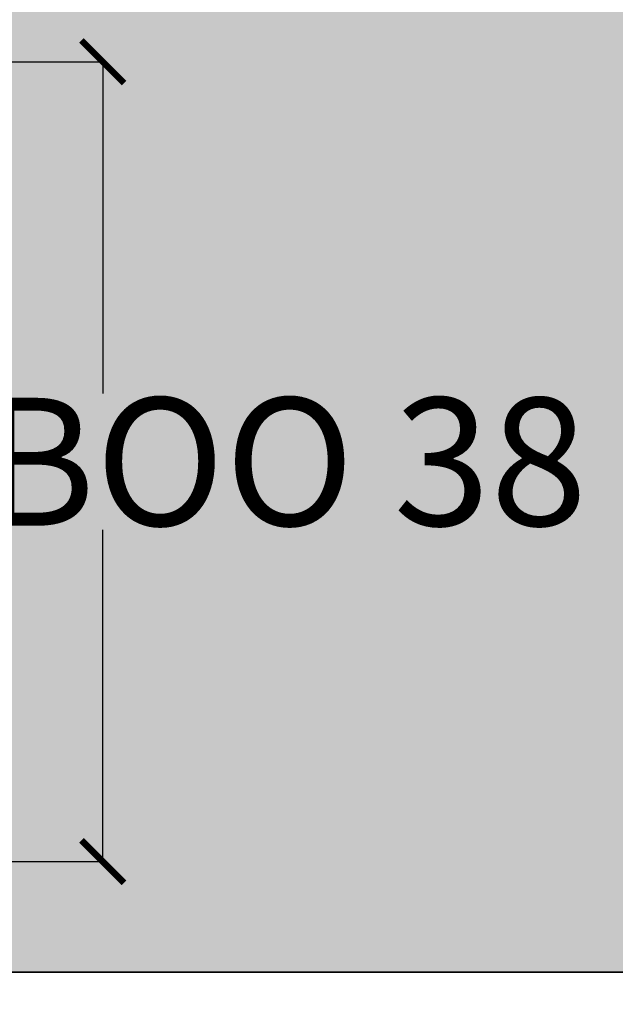
# Model space of a CAD drawing. Units: inches. Extents: x 1704 to 6393, y -157 to 1172.
# Tile 5 of 122: x 1933 to 1961, y -5 to 41. Entities that reach past the tile are written whole.
import ezdxf

# ---------------------------------------------------------------- set-up
doc = ezdxf.new("R2010")
doc.units = ezdxf.units.IN
doc.header["$MEASUREMENT"] = 0
doc.layers.add('A-ANNO-DIMS', color=7, linetype='Continuous', lineweight=13)
doc.layers.add('C-PROP', color=7, linetype='Continuous', lineweight=35)
doc.layers.add('L-PLNT-PATT', color=253, linetype='Continuous', lineweight=13, true_color=0x9abc8f)
doc.styles.get("Standard").update_dxf_attribs({"font": 'arial.ttf'})
doc.dimstyles.get("Standard").update_dxf_attribs({"dimtxt": 6, "dimasz": 2, "dimexe": 0.18, "dimexo": 0.0625, "dimgap": 0.09, "dimtad": 0, "dimtih": 1, "dimtoh": 1, "dimdec": 1, "dimzin": 0, "dimdsep": 46, "dimlunit": 3, "dimtxsty": 'Standard', "dimblk": 'ARCHTICK', "dimcen": 0.09, "dimadec": 0, "dimazin": 0, "dimtfac": 1, "dimtdec": 1, "dimtofl": 0, "dimtmove": 0, "dimatfit": 3, "dimfxl": 1, "dimtolj": 1, "dimtzin": 0, "dimarcsym": 0})

# ---------------------------------------------------------------- blocks, each defined once
blk = doc.blocks.new('_ArchTick')
at = {"color": 0, "linetype": 'ByBlock', "const_width": 0.15}
blk.add_lwpolyline([(-0.5, -0.5), (0.5, 0.5)], dxfattribs=at)
blk = doc.blocks.new('*D70')
at = {"layer": 'A-ANNO-DIMS', "color": 0, "lineweight": -2, "transparency": 16777216}
for p, q in [((1931.245, 38.926), (1936.991, 38.926)), ((1936.811, 38.926), (1936.811, 23.36)), ((1936.811, 1.402), (1936.811, 16.968)), ((1931.245, 1.402), (1936.991, 1.402))]:
    blk.add_line(p, q, dxfattribs=at)
at = {"layer": 'Defpoints', "color": 0, "lineweight": -3, "transparency": 16777216}
for p in [(1931.183, 38.926), (1931.183, 1.402), (1936.811, 1.402)]:
    blk.add_point(p, dxfattribs=at)
at = {"layer": 'A-ANNO-DIMS', "color": 0, "lineweight": -2, "transparency": 16777216, "xscale": 2, "yscale": 2, "zscale": 2}
for p, rotation in [((1936.811, 38.926), 90), ((1936.811, 1.402), 270)]:
    blk.add_blockref('_ArchTick', p, dxfattribs=dict(at, rotation=rotation))
at = {"layer": 'A-ANNO-DIMS', "color": 0, "transparency": 16777216, "insert": (1936.811, 20.164), "char_height": 6, "attachment_point": 5}
blk.add_mtext('\\A1;BAMBOO 38', dxfattribs=at)
blk = doc.blocks.new('*D90')
at = {"layer": 'A-ANNO-DIMS', "color": 0, "lineweight": -2, "transparency": 16777216}
for p, q in [((1898.349, -3.85), (1898.349, -64.967)), ((2723.349, -3.85), (2723.349, -64.967)), ((1898.349, -64.787), (2304.104, -64.787)), ((2723.349, -64.787), (2317.593, -64.787))]:
    blk.add_line(p, q, dxfattribs=at)
at = {"layer": 'Defpoints', "color": 0, "lineweight": -3, "transparency": 16777216}
for p in [(1898.349, -3.787), (2723.349, -3.787), (2723.349, -64.787)]:
    blk.add_point(p, dxfattribs=at)
at = {"layer": 'A-ANNO-DIMS', "color": 0, "lineweight": -2, "transparency": 16777216, "xscale": 2, "yscale": 2, "zscale": 2, "rotation": 180}
blk.add_blockref('_ArchTick', (1898.349, -64.787), dxfattribs=at)
at = {"layer": 'A-ANNO-DIMS', "color": 0, "lineweight": -2, "transparency": 16777216, "xscale": 2, "yscale": 2, "zscale": 2}
blk.add_blockref('_ArchTick', (2723.349, -64.787), dxfattribs=at)
at = {"layer": 'A-ANNO-DIMS', "color": 0, "transparency": 16777216, "insert": (2310.849, -64.787), "char_height": 6, "attachment_point": 5}
blk.add_mtext('\\A1;825', dxfattribs=at)

msp = doc.modelspace()

# ---------------------------------------------------------------- hatches: boundary and pattern name
at = {"layer": 'L-PLNT-PATT', "transparency": 33554643}
h = msp.add_hatch(color=256, dxfattribs=at)
h.dxf.hatch_style = 1
h.paths.add_polyline_path([(1975.349, 202.213), (1898.349, 202.213), (1898.349, -3.787), (1975.349, -3.787)])

# ---------------------------------------------------------------- linework, layer by layer
at = {"layer": 'C-PROP'}
msp.add_line((2723.349, -3.787), (1898.349, -3.787), dxfattribs=at)

# ---------------------------------------------------------------- dimensions: what is measured, and where the dimension line sits
at = {"layer": 'A-ANNO-DIMS'}
dim = msp.add_linear_dim(base=(1936.811, 1.402), p1=(1931.183, 38.926), p2=(1931.183, 1.402), angle=270, text='BAMBOO <>', dimstyle='Standard', override={"dimdec": 0, "dimlfac": 1, "dimrnd": 0, "dimzin": 0, "dimdsep": 46, "dimlunit": 2}, dxfattribs=at)
dim.commit()
dim.dimension.update_dxf_attribs({"geometry": '*D70', "text_midpoint": (1936.811, 20.164)})
dim = msp.add_linear_dim(base=(2723.349, -64.787), p1=(1898.349, -3.787), p2=(2723.349, -3.787), dimstyle='Standard', override={"dimdec": 0, "dimlfac": 1, "dimrnd": 0, "dimzin": 0, "dimdsep": 46, "dimlunit": 2}, dxfattribs=at)
dim.commit()
dim.dimension.update_dxf_attribs({"geometry": '*D90', "text_midpoint": (2310.849, -64.787)})

doc.saveas('drawing.dxf')
